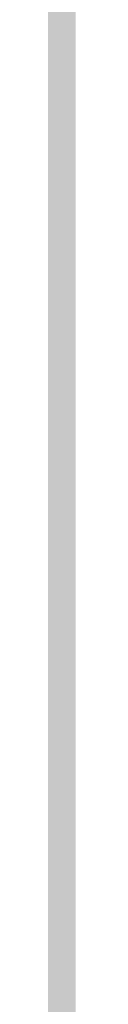
# Model space of a CAD drawing. Units: inches. Extents: x 2083 to 3317, y 1141 to 2115.
# Tile 208 of 256: x 3126.939 to 3126.956, y 1264.131 to 1265.165. Entities that reach past the tile are written whole.
import ezdxf

# ---------------------------------------------------------------- set-up
doc = ezdxf.new("R2010")
doc.units = ezdxf.units.IN
doc.layers.add('A-ANNO-DIMS', color=2, linetype='Continuous', lineweight=18)
doc.layers.add('A-WALL-PATT', color=251, linetype='Continuous', lineweight=13, true_color=0x636466)
doc.styles.get("Standard").update_dxf_attribs({"font": 'arial.ttf'})
doc.dimstyles.new('ISO-25', dxfattribs={"dimtxt": 12, "dimasz": 12, "dimexe": 1.25, "dimexo": 0.625, "dimtad": 1, "dimlunit": 3, "dimtxsty": 'Standard', "dimcen": 2.5, "dimadec": 0, "dimazin": 0, "dimtfac": 1, "dimtmove": 0, "dimatfit": 3, "dimfxl": 1, "dimarcsym": 0})

# ---------------------------------------------------------------- blocks, each defined once
blk = doc.blocks.new('*D26')
at = {"layer": 'A-ANNO-DIMS', "color": 0, "lineweight": -2, "transparency": 16777216}
for p, q in [((3088.9858, 1274.9151), (3088.9858, 1270.952)), ((3111.24, 1274.9151), (3111.24, 1270.952)), ((3076.9858, 1272.202), (2840.2624, 1272.202)), ((3111.24, 1272.202), (3088.9858, 1272.202)), ((3123.24, 1272.202), (3135.24, 1272.202))]:
    blk.add_line(p, q, dxfattribs=at)
at = {"layer": 'A-ANNO-DIMS', "color": 0, "transparency": 16777216}
for points in [[(3076.9858, 1274.202), (3076.9858, 1270.202), (3088.9858, 1272.202)], [(3123.24, 1274.202), (3123.24, 1270.202), (3111.24, 1272.202)]]:
    blk.add_solid(points, dxfattribs=at)
at = {"layer": 'Defpoints', "color": 0, "transparency": 16777216}
for p in [(3088.9858, 1275.5401), (3111.24, 1275.5401), (3088.9858, 1272.202)]:
    blk.add_point(p, dxfattribs=at)
at = {"layer": 'A-ANNO-DIMS', "color": 0, "transparency": 16777216, "insert": (2952.6241, 1279.0316), "char_height": 12, "attachment_point": 5}
blk.add_mtext('NIGHTSTAND 1\'-10 1/2" TYP.', dxfattribs=at)
blk = doc.blocks.new('*D27')
at = {"layer": 'A-ANNO-DIMS', "color": 0, "lineweight": -2, "transparency": 16777216}
for p, q in [((3114.5782, 1309.7943), (3114.5782, 1321.7943)), ((3111.865, 1297.7943), (3115.8282, 1297.7943)), ((3114.5782, 1297.7943), (3114.5782, 1275.5401)), ((3111.865, 1275.5401), (3115.8282, 1275.5401)), ((3114.5782, 1263.5401), (3114.5782, 1140.9886))]:
    blk.add_line(p, q, dxfattribs=at)
at = {"layer": 'A-ANNO-DIMS', "color": 0, "transparency": 16777216}
for points in [[(3112.5782, 1309.7943), (3116.5782, 1309.7943), (3114.5782, 1297.7943)], [(3112.5782, 1263.5401), (3116.5782, 1263.5401), (3114.5782, 1275.5401)]]:
    blk.add_solid(points, dxfattribs=at)
at = {"layer": 'Defpoints', "color": 0, "transparency": 16777216}
for p in [(3111.24, 1297.7943), (3111.24, 1275.5401), (3114.5782, 1275.5401)]:
    blk.add_point(p, dxfattribs=at)
at = {"layer": 'A-ANNO-DIMS', "color": 0, "transparency": 16777216, "insert": (3107.7485, 1196.2643), "char_height": 12, "attachment_point": 5, "rotation": 90}
blk.add_mtext('1\'-10 1/2" TYP.', dxfattribs=at)

msp = doc.modelspace()

# ---------------------------------------------------------------- hatches: boundary and pattern name
at = {"layer": 'A-WALL-PATT'}
h = msp.add_hatch(color=256, dxfattribs=at)
h.dxf.hatch_style = 1
h.paths.add_polyline_path([(3126.9598, 2020.7614), (2748.9598, 2020.7614), (2604.9598, 2020.7614), (2226.9598, 2020.7614), (2226.9598, 1702.7614), (2466.9598, 1702.7614), (2466.9598, 1582.7614), (2418.9598, 1582.7614), (2418.9598, 1477.7614), (2226.9598, 1477.7614), (2226.9598, 1263.2614), (2544.9598, 1263.2614), (2544.9598, 1411.7614), (2604.9598, 1411.7614), (2685.9598, 1411.7614), (2685.9598, 1420.7614), (2604.9598, 1420.7614), (2604.9598, 1573.7614), (2604.9598, 1702.7614), (2604.9598, 2011.7614), (2748.9598, 2011.7614), (2748.9598, 1702.7614), (2862.9598, 1702.7614), (2862.9598, 1621.7614), (2871.9598, 1621.7614), (2871.9598, 1702.7614), (2883.9598, 1702.7614), (2883.9598, 1706.9395, -0.026459), (2883.9598, 1711.7614), (2757.9598, 1711.7614), (2757.9598, 1807.7614), (2787.9598, 1807.7614), (2787.9598, 1812.2614), (2757.9598, 1812.2614), (2757.9598, 2011.7614), (2877.9598, 2011.7614), (2877.9598, 1812.2614), (2847.9598, 1812.2614), (2847.9598, 1807.7614), (2889.8357, 1807.7614), (2889.8357, 1812.2614), (2882.4598, 1812.2614), (2882.4598, 2011.7614), (3117.9598, 2011.7614), (3117.9598, 1812.2614), (2937.8357, 1812.2614), (2937.8357, 1807.7614), (2995.7098, 1807.7614), (2995.7098, 1796.1177), (3000.2098, 1796.1177), (3000.2098, 1807.7614), (3117.9598, 1807.7614), (3117.9598, 1711.7614), (3000.2098, 1711.7614), (3000.2098, 1760.1177), (2998.5727, 1760.1177, -0.020711), (2995.7098, 1760.1177), (2995.7098, 1711.7614), (2931.9598, 1711.7614), (2931.9598, 1702.7614), (3126.9598, 1702.7614)])
h.paths.add_polyline_path([(2471.4598, 2011.7614), (2471.4598, 1810.0114), (2462.7169, 1810.0114), (2462.7169, 1805.5114), (2505.9598, 1805.5114), (2505.9598, 1810.0114), (2475.9598, 1810.0114), (2475.9598, 2011.7614), (2595.9598, 2011.7614), (2595.9598, 1810.0114), (2565.9598, 1810.0114), (2565.9598, 1805.5114), (2595.9598, 1805.5114), (2595.9598, 1711.7614), (2235.9598, 1711.7614), (2235.9598, 1805.5114), (2353.7098, 1805.5114), (2353.7098, 1796.0542), (2358.2098, 1796.0542), (2358.2098, 1805.5114), (2414.7169, 1805.5114), (2414.7169, 1810.0114), (2235.9598, 1810.0114), (2235.9598, 2011.7614)], flags=16)
h.paths.add_polyline_path([(2270.2047, 1994.61), (2270.2047, 1970.61), (2246.2047, 1970.61), (2246.2047, 1994.61)], flags=0)
edge = h.paths.add_edge_path(flags=0)
edge.add_ellipse((2332.0274, 1899.7982), major_axis=(-3.043, 3.043), ratio=0.168252, start_angle=-161.3322, end_angle=-156.3071, ccw=False)
edge.add_ellipse((2333.082, 1898.7435), major_axis=(-1.0546, 1.0546), ratio=0.453532, start_angle=-123.371, end_angle=-94.1591)
edge = h.paths.add_edge_path(flags=0)
edge.add_ellipse((2332.0274, 1968.8763), major_axis=(3.043, 3.043), ratio=0.168252, start_angle=18.6678, end_angle=23.6929)
edge.add_spline(control_points=[(2332.9256, 1970.6911), (2332.2268, 1970.3361), (2330.8937, 1969.6589), (2328.4131, 1970.9321), (2327.2039, 1967.7487), (2324.7096, 1969.9556), (2322.5328, 1967.0124), (2320.0128, 1971.2958), (2317.6803, 1968.1578), (2316.0405, 1967.102), (2315.4269, 1966.8096)], knot_values=[0, 0, 0, 0, 2.267059, 4.324559, 6.685584, 8.878641, 11.121502, 14.300359, 17.755284, 19.732645, 19.732645, 19.732645, 19.732645], degree=3, periodic=0)
edge.add_ellipse((2332.0274, 1968.8763), major_axis=(3.043, 3.043), ratio=0.168252, start_angle=18.6678, end_angle=23.6929, ccw=False)
edge.add_ellipse((2333.082, 1969.9309), major_axis=(1.0546, 1.0546), ratio=0.453532, start_angle=56.629, end_angle=85.8409, ccw=False)
edge = h.paths.add_edge_path(flags=0)
edge.add_spline(control_points=[(2296.4283, 1967.9879), (2293.6278, 1965.3363), (2287.7036, 1959.7271), (2299.7439, 1949.9957), (2294.5326, 1935.6685), (2290.5732, 1920.6035), (2293.3941, 1909.9737), (2296.1854, 1904.9665)], knot_values=[0.099185, 0.099185, 0.099185, 0.099185, 0.345301, 0.619822, 0.982653, 1.386093, 1.810555, 1.810555, 1.810555, 1.810555], degree=3, periodic=0)
edge.add_spline(control_points=[(2296.1854, 1904.9665), (2297.3836, 1902.6193), (2298.001, 1901.9493), (2298.553, 1901.4682)], knot_values=[0.006246, 0.006246, 0.006246, 0.006246, 0.055476, 0.055476, 0.055476, 0.055476], degree=3, periodic=0)
edge.add_spline(control_points=[(2298.553, 1901.4682), (2297.2586, 1900.9232), (2295.2253, 1900.2321), (2293.0602, 1900.6142), (2292.1014, 1900.7884), (2292.0896, 1900.7906)], knot_values=[0.312835, 0.312835, 0.312835, 0.312835, 0.40178, 0.474987, 0.475903, 0.475903, 0.475903, 0.475903], degree=3, periodic=0)
edge.add_arc((2292.7936, 1904.6641), 3.937, 215.4209, 259.6982, ccw=False)
edge.add_spline(control_points=[(2289.5853, 1902.3823), (2289.4767, 1902.5351), (2289.3685, 1902.688), (2289.2609, 1902.8412)], knot_values=[0.102872, 0.102872, 0.102872, 0.102872, 0.116896, 0.116896, 0.116896, 0.116896], degree=3, periodic=0)
edge.add_spline(control_points=[(2289.2609, 1902.8412), (2288.6866, 1902.5502), (2287.64, 1902.0199), (2285.8813, 1901.874), (2283.853, 1901.5044), (2281.72, 1899.7105), (2278.467, 1899.4929), (2276.1571, 1901.8832), (2272.259, 1899.8041), (2267.7776, 1901.8432), (2262.2439, 1900.184), (2257.4149, 1901.7821), (2254.3184, 1900.7261), (2253.1783, 1900.3373)], knot_values=[0, 0, 0, 0, 1.907977, 3.477176, 5.261074, 7.972851, 11.680248, 13.717921, 16.939592, 22.789562, 27.502503, 33.595215, 37.145618, 37.145618, 37.145618, 37.145618], degree=3, periodic=0)
edge.add_line((2253.1783, 1900.3373), (2250.2442, 1902.8412))
edge.add_line((2250.2442, 1902.8412), (2250.2442, 1965.8333))
edge.add_line((2250.2442, 1965.8333), (2253.1783, 1968.3371))
edge.add_spline(control_points=[(2253.1783, 1968.3371), (2254.3184, 1967.9483), (2257.4149, 1966.8924), (2262.2439, 1968.4904), (2267.7776, 1966.8313), (2271.5267, 1968.5372), (2273.8759, 1967.8283), (2274.2067, 1967.7276)], knot_values=[0, 0, 0, 0, 0.09018, 0.244935, 0.364644, 0.513233, 0.537855, 0.537855, 0.537855, 0.537855], degree=3, periodic=0)
edge.add_arc((2274.3529, 1963.7933), 3.937, 72.0511, 92.1279, ccw=False)
edge.add_arc((2281.2969, 1985.23), 18.5963, 252.05113, 288.56572)
edge.add_arc((2292.3167, 1956.0289), 12.6461, 71.02679, 113.77822, ccw=False)
edge = h.paths.add_edge_path(flags=0)
edge.add_spline(control_points=[(2274.8994, 1951.8562), (2275.0662, 1951.6166), (2275.2327, 1951.3766), (2275.398, 1951.1359)], knot_values=[1.409916, 1.409916, 1.409916, 1.409916, 1.43159, 1.43159, 1.43159, 1.43159], degree=3, periodic=0)
edge.add_spline(control_points=[(2275.398, 1951.1359), (2275.7921, 1950.5619), (2276.1792, 1949.9838), (2276.5455, 1949.3971)], knot_values=[1.358238, 1.358238, 1.358238, 1.358238, 1.409916, 1.409916, 1.409916, 1.409916], degree=3, periodic=0)
edge.add_line((2276.5455, 1949.3971), (2277.4373, 1947.8622))
edge.add_spline(control_points=[(2277.4373, 1947.8622), (2276.3038, 1945.6731), (2274.6397, 1942.4269), (2274.6316, 1938.0939), (2272.7991, 1930.8515), (2274.3564, 1943.897), (2275.9477, 1947.9234), (2276.5455, 1949.3971)], knot_values=[0.005632, 0.005632, 0.005632, 0.005632, 0.186014, 0.266002, 0.357087, 0.59639, 0.739732, 0.739732, 0.739732, 0.739732], degree=3, periodic=0)
edge.add_spline(control_points=[(2276.5455, 1949.3971), (2276.1792, 1949.9838), (2275.7921, 1950.5619), (2275.398, 1951.1359)], knot_values=[1.358238, 1.358238, 1.358238, 1.358238, 1.409916, 1.409916, 1.409916, 1.409916], degree=3, periodic=0)
edge.add_spline(control_points=[(2275.398, 1951.1359), (2274.9425, 1950.0805), (2274.2078, 1948.0253), (2273.9346, 1944.8515), (2272.4685, 1937.6275), (2273.4662, 1945.6965), (2274.7006, 1951.0595), (2274.8994, 1951.8562)], knot_values=[0.104364, 0.104364, 0.104364, 0.104364, 0.189636, 0.269624, 0.36071, 0.600013, 0.644622, 0.644622, 0.644622, 0.644622], degree=3, periodic=0)
h.paths.add_polyline_path([(2269.1675, 1963.1276, -0.357527), (2268.1706, 1960.9764, -0.092561), (2268.1706, 1939.4363, -0.357527), (2269.1675, 1937.2851, -0.357527), (2267.0163, 1938.282, -0.164785), (2254.6856, 1938.282, -0.357527), (2252.5344, 1937.2851, -0.357527), (2253.5313, 1939.4363, -0.092561), (2253.5313, 1960.9764, -0.357527), (2252.5344, 1963.1276, -0.357527), (2254.6856, 1962.1307, -0.164785), (2267.0163, 1962.1307, -0.357527)], flags=0)
h.paths.add_polyline_path([(2248.8741, 1967.8018), (2248.8741, 1957.0277), (2249.4578, 1957.0277), (2249.4578, 1911.6468), (2248.8741, 1911.6468), (2248.8741, 1900.8727), (2246.5119, 1900.8727, 0.197327), (2244.1497, 1902.4569), (2244.1497, 1966.2176, 0.197327), (2246.5119, 1967.8018)], flags=0)
h.paths.add_polyline_path([(2269.1675, 1931.3893, -0.357527), (2268.1706, 1929.2381, -0.092561), (2268.1706, 1907.6981, -0.357527), (2269.1675, 1905.5469, -0.357527), (2267.0163, 1906.5438, -0.164785), (2254.6856, 1906.5438, -0.357527), (2252.5344, 1905.5469, -0.357527), (2253.5313, 1907.6981, -0.092561), (2253.5313, 1929.2381, -0.357527), (2252.5344, 1931.3893, -0.357527), (2254.6856, 1930.3925, -0.164785), (2267.0163, 1930.3925, -0.357527)], flags=0)
edge = h.paths.add_edge_path(flags=0)
edge.add_spline(control_points=[(2276.1969, 1906.7237), (2276.1681, 1909.0289), (2276.114, 1913.3719), (2270.5984, 1924.925), (2273.9052, 1919.0128), (2275.9217, 1916.2621), (2275.4746, 1912.4021), (2277.2579, 1910.3806), (2276.696, 1908.225), (2276.6462, 1906.813), (2276.6178, 1906.0084)], knot_values=[0, 0, 0, 0, 8.61026, 16.221274, 18.843057, 23.804898, 27.440828, 29.356102, 31.203478, 33.650687, 33.650687, 33.650687, 33.650687], degree=3, periodic=0)
edge.add_spline(control_points=[(2276.6178, 1906.0084), (2276.6233, 1905.6241), (2276.4977, 1904.6287), (2275.4418, 1903.8547), (2274.9373, 1903.0804), (2274.8591, 1902.8412)], knot_values=[0.156488, 0.156488, 0.156488, 0.156488, 0.184398, 0.231376, 0.250598, 0.250598, 0.250598, 0.250598], degree=3, periodic=0)
edge.add_line((2274.8591, 1902.8412), (2276.506, 1902.8412))
edge.add_spline(control_points=[(2276.506, 1902.8412), (2276.7883, 1903.0849), (2277.6651, 1904.1252), (2278.2495, 1904.3407), (2277.6539, 1908.5274), (2278.1557, 1906.2278), (2278.1005, 1905.2859), (2278.8467, 1904.069), (2277.8568, 1903.4149), (2277.8742, 1902.991), (2277.9036, 1902.8412)], knot_values=[0.059574, 0.059574, 0.059574, 0.059574, 0.080753, 0.103741, 0.16972, 0.176036, 0.207137, 0.240474, 0.262341, 0.27366, 0.27366, 0.27366, 0.27366], degree=3, periodic=0)
edge.add_line((2277.9036, 1902.8412), (2280.0298, 1902.8412))
edge.add_spline(control_points=[(2280.0298, 1902.8412), (2279.8882, 1903.0884), (2279.4993, 1903.9816), (2280.1523, 1905.9393), (2278.1036, 1909.6578), (2279.7624, 1907.1853), (2280.3279, 1904.8749), (2280.4851, 1903.4896), (2281.4633, 1903.2494), (2281.7583, 1902.9365), (2281.834, 1902.8412)], knot_values=[0.013856, 0.013856, 0.013856, 0.013856, 0.034874, 0.088867, 0.107879, 0.126738, 0.158714, 0.193757, 0.217487, 0.226722, 0.226722, 0.226722, 0.226722], degree=3, periodic=0)
edge.add_spline(control_points=[(2281.834, 1902.8412), (2281.7875, 1902.8267), (2281.647, 1902.783), (2281.3955, 1902.8595), (2281.0881, 1902.9852), (2280.7207, 1903.0609), (2280.3335, 1903.0257), (2280.1248, 1902.8989), (2280.0298, 1902.8412)], knot_values=[0, 0, 0, 0, 0.14413, 0.435517, 0.749276, 1.153046, 1.548371, 1.878348, 1.878348, 1.878348, 1.878348], degree=3, periodic=0)
edge.add_line((2280.0298, 1902.8412), (2277.9036, 1902.8412))
edge.add_spline(control_points=[(2277.9036, 1902.8412), (2277.8929, 1902.7959), (2277.8654, 1902.6796), (2277.6075, 1902.6875), (2277.2741, 1902.8007), (2276.8379, 1902.6198), (2276.5838, 1902.7893), (2276.506, 1902.8412)], knot_values=[0, 0, 0, 0, 0.127189, 0.326199, 0.628009, 1.24357, 1.515331, 1.515331, 1.515331, 1.515331], degree=3, periodic=0)
edge.add_line((2276.506, 1902.8412), (2274.8591, 1902.8412))
edge.add_spline(control_points=[(2274.8591, 1902.8412), (2274.8144, 1902.8986), (2274.7251, 1903.0134), (2274.4935, 1903.119), (2274.2443, 1902.9605), (2273.9371, 1903.1849), (2273.614, 1902.9831), (2273.4083, 1902.883), (2273.3223, 1902.8412)], knot_values=[0, 0, 0, 0, 0.21843, 0.436957, 0.687977, 0.990379, 1.398396, 1.69185, 1.69185, 1.69185, 1.69185], degree=3, periodic=0)
edge.add_spline(control_points=[(2273.3223, 1902.8412), (2273.6167, 1903.4457), (2274.274, 1904.5383), (2276.0272, 1904.5737), (2276.207, 1906.5836), (2276.1969, 1906.7237)], knot_values=[0.012227, 0.012227, 0.012227, 0.012227, 0.059472, 0.106218, 0.134458, 0.134458, 0.134458, 0.134458], degree=3, periodic=0)
h.paths.add_polyline_path([(2270.7761, 1897.7898), (2270.7761, 1873.7898), (2246.7761, 1873.7898), (2246.7761, 1897.7898)], flags=0)
h.paths.add_polyline_path([(2353.7098, 1760.0051), (2353.7098, 1760.0542), (2358.2098, 1760.0542, -0.033729)], flags=0)
h.paths.add_polyline_path([(2321.8191, 1737.5292), (2341.9953, 1737.5292, -0.414214), (2343.2033, 1736.3212), (2343.2033, 1721.0206, -0.414214), (2341.9953, 1719.8127), (2321.8191, 1719.8127, -0.414214), (2320.6112, 1721.0206), (2320.6112, 1736.3212, -0.414214)], flags=0)
h.paths.add_polyline_path([(2324.235, 1736.3212), (2339.5794, 1736.3212, -0.414214), (2341.9953, 1733.9053), (2341.9953, 1725.4497, -0.414214), (2339.5794, 1723.0338), (2333.6806, 1723.0338), (2333.8453, 1722.0455, -0.870646), (2335.4254, 1721.8259, -0.767327), (2333.9227, 1721.4232), (2331.291, 1721.4232, -0.767327), (2329.7883, 1721.8259, -0.870646), (2331.3684, 1722.0455), (2331.5331, 1723.0338), (2324.235, 1723.0338, -0.414214), (2321.8191, 1725.4497), (2321.8191, 1733.9053, -0.414214)], flags=0)
h.paths.add_polyline_path([(2570.4838, 1928.6154), (2589.6838, 1928.6154), (2590.1688, 1928.6154), (2590.1688, 1904.9934), (2570.4838, 1904.9934)], flags=0)
h.paths.add_polyline_path([(2574.4473, 1927.2638, -1), (2572.8288, 1927.2638, -1)], flags=0)
h.paths.add_polyline_path([(2573.0899, 1926.9409), (2573.925, 1927.776), (2574.1477, 1927.5533), (2573.3126, 1926.7182)], flags=0)
h.paths.add_polyline_path([(2578.7791, 1919.7296, -1), (2571.5917, 1919.7296, -1)], flags=0)
h.paths.add_polyline_path([(2578.3854, 1919.7296, -1), (2571.9854, 1919.7296, -1)], flags=0)
h.paths.add_polyline_path([(2331.5958, 1729.4762, -1), (2333.618, 1729.4762, -1)], flags=0)
h.paths.add_polyline_path([(2578.0342, 1927.2638, -1), (2576.4157, 1927.2638, -1)], flags=0)
h.paths.add_polyline_path([(2576.6889, 1927.5311), (2576.9116, 1927.7538), (2577.7467, 1926.9186), (2577.524, 1926.6959)], flags=0)
h.paths.add_polyline_path([(2578.1391, 1909.8595, -1), (2572.2317, 1909.8595, -1)], flags=0)
h.paths.add_polyline_path([(2577.7454, 1909.8595, -1), (2572.6254, 1909.8595, -1)], flags=0)
h.paths.add_polyline_path([(2583.7977, 1927.2638, -1), (2582.1792, 1927.2638, -1)], flags=0)
h.paths.add_polyline_path([(2582.7186, 1927.7538), (2583.5538, 1926.9186), (2583.3311, 1926.6959), (2582.4959, 1927.5311)], flags=0)
h.paths.add_polyline_path([(2582.4959, 1927.5311), (2582.7186, 1927.7538), (2583.5538, 1926.9186), (2583.3311, 1926.6959)], flags=0)
h.paths.add_polyline_path([(2587.7391, 1920.5296, -1), (2581.8317, 1920.5296, -1)], flags=0)
h.paths.add_polyline_path([(2587.3454, 1920.5296, -1), (2582.2254, 1920.5296, -1)], flags=0)
h.paths.add_polyline_path([(2587.3846, 1927.2638, -1), (2585.7661, 1927.2638, -1)], flags=0)
h.paths.add_polyline_path([(2586.082, 1926.9802), (2586.9172, 1927.8154), (2587.1399, 1927.5927), (2586.3047, 1926.7575)], flags=0)
h.paths.add_polyline_path([(2588.3791, 1910.6595, -1), (2581.1917, 1910.6595, -1)], flags=0)
h.paths.add_polyline_path([(2587.9854, 1910.6595, -1), (2581.5854, 1910.6595, -1)], flags=0)
h.paths.add_polyline_path([(2417.1677, 1729.4779), (2437.3439, 1729.4779, -0.414214), (2438.5519, 1728.2699), (2438.5519, 1712.9693, -0.414214), (2437.3439, 1711.7614), (2417.1677, 1711.7614, -0.414214), (2415.9598, 1712.9693), (2415.9598, 1728.2699, -0.414214)], flags=0)
h.paths.add_polyline_path([(2419.5836, 1728.2699), (2434.928, 1728.2699, -0.414214), (2437.3439, 1725.8541), (2437.3439, 1717.3984, -0.414214), (2434.928, 1714.9825), (2429.0292, 1714.9825), (2429.1939, 1713.9942, -0.870646), (2430.774, 1713.7746, -0.767327), (2429.2713, 1713.372), (2426.6396, 1713.372, -0.767327), (2425.1369, 1713.7746, -0.870646), (2426.717, 1713.9942), (2426.8817, 1714.9825), (2419.5836, 1714.9825, -0.414214), (2417.1677, 1717.3984), (2417.1677, 1725.8541, -0.414214)], flags=0)
h.paths.add_polyline_path([(2419.5836, 1728.2699), (2434.928, 1728.2699, -0.414214), (2437.3439, 1725.8541), (2437.3439, 1717.3984, -0.414214), (2434.928, 1714.9825), (2429.0292, 1714.9825), (2428.3581, 1719.009), (2427.5528, 1719.009), (2426.8817, 1714.9825), (2419.5836, 1714.9825, -0.414214), (2417.1677, 1717.3984), (2417.1677, 1725.8541, -0.414214)], flags=0)
h.paths.add_polyline_path([(2426.9444, 1721.4249, -1), (2428.9666, 1721.4249, -1)], flags=0)
h.paths.add_polyline_path([(2475.9598, 1702.7614), (2595.9598, 1702.7614), (2595.9598, 1582.7614), (2475.9598, 1582.7614)], flags=16)
h.paths.add_polyline_path([(2427.9598, 1573.7614), (2595.9598, 1573.7614), (2595.9598, 1468.7614), (2595.9598, 1420.7614), (2384.4598, 1420.7614), (2384.4598, 1468.7614), (2427.9598, 1468.7614)], flags=16)
h.paths.add_polyline_path([(2379.9598, 1468.7614), (2379.9598, 1420.7614), (2235.9598, 1420.7614), (2235.9598, 1468.7614)], flags=16)
h.paths.add_polyline_path([(2317.816, 1466.6958), (2337.9922, 1466.6958, -0.414214), (2339.2002, 1465.4878), (2339.2002, 1450.1872, -0.414214), (2337.9922, 1448.9792), (2317.816, 1448.9792, -0.414214), (2316.6081, 1450.1872), (2316.6081, 1465.4878, -0.414214)], flags=0)
h.paths.add_polyline_path([(2320.2319, 1465.4878), (2335.5763, 1465.4878, -0.414214), (2337.9922, 1463.0719), (2337.9922, 1454.6163, -0.414214), (2335.5763, 1452.2004), (2329.6775, 1452.2004), (2329.8422, 1451.212, -0.870646), (2331.4223, 1450.9925, -0.767327), (2329.9196, 1450.5898), (2327.2879, 1450.5898, -0.767327), (2325.7852, 1450.9925, -0.870646), (2327.3653, 1451.212), (2327.53, 1452.2004), (2320.2319, 1452.2004, -0.414214), (2317.816, 1454.6163), (2317.816, 1463.0719, -0.414214)], flags=0)
h.paths.add_polyline_path([(2320.2319, 1465.4878), (2335.5763, 1465.4878, -0.414214), (2337.9922, 1463.0719), (2337.9922, 1454.6163, -0.414214), (2335.5763, 1452.2004), (2329.6775, 1452.2004), (2329.0064, 1456.2269), (2328.2011, 1456.2269), (2327.53, 1452.2004), (2320.2319, 1452.2004, -0.414214), (2317.816, 1454.6163), (2317.816, 1463.0719, -0.414214)], flags=0)
h.paths.add_polyline_path([(2327.5926, 1458.6428, -1), (2329.6148, 1458.6428, -1)], flags=0)
h.paths.add_polyline_path([(2244.4117, 1433.3405), (2241.9209, 1433.3405, -0.414214), (2240.0179, 1435.2435), (2240.0179, 1440.9528, -0.414211), (2241.9209, 1442.8559), (2244.4117, 1442.8559, -1.976472)], flags=0)
h.paths.add_polyline_path([(2245.3569, 1434.3975, -0.414214), (2245.3569, 1441.7988, -2.144098)], flags=0)
h.paths.add_polyline_path([(2535.9598, 1416.2614), (2535.9598, 1272.2614), (2235.9598, 1272.2614), (2235.9598, 1416.2614)], flags=16)
h.paths.add_polyline_path([(2260.1196, 1384.2928), (2260.1196, 1362.0386), (2237.8654, 1362.0386), (2237.8654, 1384.2928)], flags=0)
edge = h.paths.add_edge_path(flags=0)
edge.add_line((2318.2518, 1362.0933), (2318.1458, 1362.001))
edge.add_ellipse((2317.4451, 1360.431), major_axis=(2.8216, 2.8216), ratio=0.168252, start_angle=18.6678, end_angle=20.9481, ccw=False)
edge.add_ellipse((2318.423, 1361.409), major_axis=(0.9779, 0.9779), ratio=0.453532, start_angle=56.629, end_angle=70.2262, ccw=False)
edge = h.paths.add_edge_path(flags=0)
edge.add_line((2319.1074, 1295.5711), (2319.015, 1295.6771))
edge.add_ellipse((2317.4451, 1296.3778), major_axis=(-2.8216, 2.8216), ratio=0.168252, start_angle=-161.3322, end_angle=-159.0519, ccw=False)
edge.add_ellipse((2318.423, 1295.3999), major_axis=(-0.9779, 0.9779), ratio=0.453532, start_angle=-123.371, end_angle=-109.7738)
edge = h.paths.add_edge_path(flags=0)
edge.add_spline(control_points=[(2284.2103, 1301.1702), (2284.5807, 1300.4447), (2284.8912, 1299.892), (2285.1596, 1299.461)], knot_values=[0.039066, 0.039066, 0.039066, 0.039066, 0.055476, 0.055476, 0.055476, 0.055476], degree=3, periodic=0)
edge.add_line((2285.1596, 1299.461), (2284.2103, 1301.1702))
edge = h.paths.add_edge_path(flags=0)
edge.add_line((2280.4125, 1297.298), (2283.37, 1297.0361))
edge.add_line((2283.37, 1297.0361), (2286.4057, 1297.9263))
edge.add_spline(control_points=[(2286.4057, 1297.9263), (2285.3055, 1297.4631), (2284.3448, 1297.1292), (2283.37, 1297.0361)], knot_values=[0.394369, 0.394369, 0.394369, 0.394369, 0.475903, 0.475903, 0.475903, 0.475903], degree=3, periodic=0)
edge.add_spline(control_points=[(2283.37, 1297.0361), (2283.2814, 1297.0277), (2282.3163, 1296.9573), (2281.3125, 1297.1345), (2280.4234, 1297.296), (2280.4125, 1297.298)], knot_values=[0.312835, 0.312835, 0.312835, 0.312835, 0.320246, 0.393453, 0.394369, 0.394369, 0.394369, 0.394369], degree=3, periodic=0)
edge = h.paths.add_edge_path(flags=0)
edge.add_line((2284.4356, 1359.6073), (2280.4463, 1355.328))
edge.add_line((2280.4463, 1355.328), (2279.58, 1351.0178))
edge.add_line((2279.58, 1351.0178), (2282.413, 1346.5804))
edge.add_spline(control_points=[(2282.413, 1346.5804), (2283.1533, 1345.5892), (2284.2529, 1344.0289), (2284.801, 1342.3872), (2284.9352, 1341.8055)], knot_values=[1.240098, 1.240098, 1.240098, 1.240098, 1.332892, 1.382712, 1.382712, 1.382712, 1.382712], degree=3, periodic=0)
edge.add_spline(control_points=[(2284.9352, 1341.8055), (2285.3191, 1340.1406), (2285.233, 1338.4092), (2284.9099, 1336.6541)], knot_values=[1.097484, 1.097484, 1.097484, 1.097484, 1.240098, 1.240098, 1.240098, 1.240098], degree=3, periodic=0)
edge.add_spline(control_points=[(2284.9099, 1336.6541), (2284.5868, 1334.899), (2284.0267, 1333.1203), (2283.4626, 1331.3606)], knot_values=[0.95487, 0.95487, 0.95487, 0.95487, 1.097484, 1.097484, 1.097484, 1.097484], degree=3, periodic=0)
edge.add_line((2283.4626, 1331.3606), (2281.8904, 1326.1534))
edge.add_line((2281.8904, 1326.1534), (2280.7563, 1321.0561))
edge.add_line((2280.7563, 1321.0561), (2280.2992, 1316.002))
edge.add_line((2280.2992, 1316.002), (2280.7159, 1310.9501))
edge.add_line((2280.7159, 1310.9501), (2282.0281, 1305.9721))
edge.add_line((2282.0281, 1305.9721), (2284.2103, 1301.1702))
edge.add_spline(control_points=[(2284.2103, 1301.1702), (2283.3407, 1302.7302), (2282.6119, 1304.3365), (2282.0281, 1305.9721)], knot_values=[0.099185, 0.099185, 0.099185, 0.099185, 0.241799, 0.241799, 0.241799, 0.241799], degree=3, periodic=0)
edge.add_spline(control_points=[(2282.0281, 1305.9721), (2281.4443, 1307.6078), (2281.0055, 1309.2728), (2280.7159, 1310.9501)], knot_values=[0.241799, 0.241799, 0.241799, 0.241799, 0.384413, 0.384413, 0.384413, 0.384413], degree=3, periodic=0)
edge.add_spline(control_points=[(2280.7159, 1310.9501), (2280.4332, 1312.5876), (2280.2894, 1314.277), (2280.2989, 1315.962), (2280.2992, 1316.002)], knot_values=[0.384413, 0.384413, 0.384413, 0.384413, 0.523647, 0.527028, 0.527028, 0.527028, 0.527028], degree=3, periodic=0)
edge.add_spline(control_points=[(2280.2992, 1316.002), (2280.3123, 1317.687), (2280.4779, 1319.3679), (2280.7563, 1321.0561)], knot_values=[0.527028, 0.527028, 0.527028, 0.527028, 0.669642, 0.669642, 0.669642, 0.669642], degree=3, periodic=0)
edge.add_spline(control_points=[(2280.7563, 1321.0561), (2281.0346, 1322.7443), (2281.4259, 1324.4396), (2281.8904, 1326.1534)], knot_values=[0.669642, 0.669642, 0.669642, 0.669642, 0.812256, 0.812256, 0.812256, 0.812256], degree=3, periodic=0)
edge.add_spline(control_points=[(2281.8904, 1326.1534), (2282.2644, 1327.5333), (2282.7879, 1329.2618), (2283.3528, 1331.0178), (2283.4626, 1331.3606)], knot_values=[0.812256, 0.812256, 0.812256, 0.812256, 0.927087, 0.95487, 0.95487, 0.95487, 0.95487], degree=3, periodic=0)
edge.add_line((2283.4626, 1331.3606), (2284.9099, 1336.6541))
edge.add_line((2284.9099, 1336.6541), (2284.9352, 1341.8055))
edge.add_line((2284.9352, 1341.8055), (2282.413, 1346.5804))
edge.add_spline(control_points=[(2282.413, 1346.5804), (2281.2751, 1348.1038), (2280.0784, 1349.5703), (2279.58, 1351.0178)], knot_values=[1.382712, 1.382712, 1.382712, 1.382712, 1.525326, 1.525326, 1.525326, 1.525326], degree=3, periodic=0)
edge.add_spline(control_points=[(2279.58, 1351.0178), (2279.4433, 1351.4147), (2279.1363, 1352.8569), (2279.7352, 1354.2904), (2280.4463, 1355.328)], knot_values=[1.525326, 1.525326, 1.525326, 1.525326, 1.564439, 1.667941, 1.667941, 1.667941, 1.667941], degree=3, periodic=0)
edge.add_spline(control_points=[(2280.4463, 1355.328), (2281.4261, 1356.7578), (2282.9308, 1358.1826), (2284.4356, 1359.6073)], knot_values=[1.667941, 1.667941, 1.667941, 1.667941, 1.810555, 1.810555, 1.810555, 1.810555], degree=3, periodic=0)
edge.add_arc((2280.6231, 1348.5182), 11.7262, 71.02679, 113.77822)
edge.add_arc((2270.4049, 1375.5952), 17.2436, 252.05113, 288.56572, ccw=False)
edge.add_arc((2263.966, 1355.7178), 3.6506, 72.0511, 92.1279)
edge.add_arc((2263.966, 1355.7178), 3.6506, 92.1279, 177.9851)
edge.add_spline(control_points=[(2260.3176, 1355.8462), (2260.2604, 1354.2207), (2260.5513, 1350.1865), (2262.9993, 1346.7663), (2264.4727, 1344.649)], knot_values=[1.43159, 1.43159, 1.43159, 1.43159, 1.564144, 1.770695, 1.770695, 1.770695, 1.770695], degree=3, periodic=0)
edge.add_line((2264.4727, 1344.649), (2264.9356, 1343.9825))
edge.add_spline(control_points=[(2263.801, 1340.2481), (2263.8432, 1340.5141), (2264.0672, 1341.7565), (2264.5127, 1343.0025), (2264.935, 1343.9811)], knot_values=[0.53657, 0.53657, 0.53657, 0.53657, 0.559349, 0.644622, 0.644622, 0.644622, 0.644622], degree=3, periodic=0)
edge.add_spline(control_points=[(2264.935, 1343.9811), (2265.1178, 1343.715), (2265.2989, 1343.4479), (2265.4768, 1343.1794)], knot_values=[1.384077, 1.384077, 1.384077, 1.384077, 1.409916, 1.409916, 1.409916, 1.409916], degree=3, periodic=0)
edge.add_spline(control_points=[(2265.4768, 1343.1794), (2265.6546, 1342.9108), (2265.8293, 1342.6408), (2265.9991, 1342.3688)], knot_values=[1.358238, 1.358238, 1.358238, 1.358238, 1.384077, 1.384077, 1.384077, 1.384077], degree=3, periodic=0)
edge.add_line((2265.9991, 1342.3688), (2266.826, 1340.9455))
edge.add_spline(control_points=[(2266.826, 1340.9455), (2268.8944, 1337.0897), (2271.3982, 1325.843), (2270.5162, 1310.5686), (2275.9194, 1301.8606), (2277.7895, 1299.1994)], knot_values=[0.116896, 0.116896, 0.116896, 0.116896, 0.472987, 1.050969, 1.313793, 1.313793, 1.313793, 1.313793], degree=3, periodic=0)
edge.add_spline(control_points=[(2277.7895, 1299.1994), (2277.8394, 1299.1285), (2277.8894, 1299.0575), (2277.9396, 1298.9866)], knot_values=[0.109884, 0.109884, 0.109884, 0.109884, 0.116896, 0.116896, 0.116896, 0.116896], degree=3, periodic=0)
edge.add_line((2277.9396, 1298.9866), (2277.7888, 1299.1991))
edge.add_spline(control_points=[(2277.7888, 1299.1991), (2277.2566, 1298.9294), (2276.2864, 1298.4379), (2275.0394, 1298.3344), (2274.3833, 1298.2389), (2274.2153, 1298.2093)], knot_values=[33.12187, 33.12187, 33.12187, 33.12187, 35.029056, 36.598255, 37.144827, 37.144827, 37.144827, 37.144827], degree=3, periodic=0)
edge.add_line((2274.2153, 1298.2093), (2273.0731, 1297.893))
edge.add_spline(control_points=[(2273.0731, 1297.893), (2272.3229, 1297.5798), (2271.0392, 1296.5105), (2269.2484, 1296.2261), (2268.4231, 1296.3747)], knot_values=[26.532584, 26.532584, 26.532584, 26.532584, 29.198919, 31.839101, 31.839101, 31.839101, 31.839101], degree=3, periodic=0)
edge.add_line((2268.4231, 1296.3747), (2263.8785, 1297.4575))
edge.add_spline(control_points=[(2263.8785, 1297.4575), (2263.5561, 1297.3594), (2261.8603, 1296.8387), (2260.2388, 1297.2824), (2258.9335, 1297.5165)], knot_values=[15.919551, 15.919551, 15.919551, 15.919551, 16.939592, 21.226067, 21.226067, 21.226067, 21.226067], degree=3, periodic=0)
edge.add_line((2258.9335, 1297.5165), (2254.0552, 1297.329))
edge.add_spline(control_points=[(2254.0552, 1297.329), (2253.7555, 1297.2958), (2252.1137, 1297.1652), (2250.4619, 1297.5442), (2249.1297, 1297.6679)], knot_values=[5.306517, 5.306517, 5.306517, 5.306517, 6.276435, 10.613034, 10.613034, 10.613034, 10.613034], degree=3, periodic=0)
edge.add_line((2249.1297, 1297.6679), (2244.3316, 1296.8778))
edge.add_line((2244.3316, 1296.8778), (2241.611, 1299.1994))
edge.add_line((2241.611, 1299.1994), (2241.611, 1357.6094))
edge.add_line((2241.611, 1357.6094), (2244.3316, 1359.9311))
edge.add_line((2244.3316, 1359.9311), (2252.7288, 1359.5427))
edge.add_spline(control_points=[(2252.7288, 1359.5427), (2252.8709, 1359.5464), (2253.3057, 1359.5482), (2253.7398, 1359.5143), (2254.0317, 1359.4824)], knot_values=[0.233291, 0.233291, 0.233291, 0.233291, 0.244935, 0.268927, 0.268927, 0.268927, 0.268927], degree=3, periodic=0)
edge.add_line((2254.0317, 1359.4824), (2259.5872, 1359.4164))
edge.add_spline(control_points=[(2259.5872, 1359.4164), (2260.6771, 1359.6285), (2262.0732, 1359.897), (2263.5237, 1359.4593), (2263.8304, 1359.366)], knot_values=[0.422516, 0.422516, 0.422516, 0.422516, 0.513233, 0.537855, 0.537855, 0.537855, 0.537855], degree=3, periodic=0)
edge.add_arc((2263.966, 1355.7178), 3.6506, 72.0511, 92.1279, ccw=False)
edge.add_arc((2270.4049, 1375.5952), 17.2436, 252.05113, 288.56572)
edge.add_arc((2280.6231, 1348.5182), 11.7262, 71.02679, 113.77822, ccw=False)
h.paths.add_polyline_path([(2240.3405, 1359.4347), (2240.3405, 1349.4444), (2240.8818, 1349.4444), (2240.8818, 1307.3645), (2240.3405, 1307.3645), (2240.3405, 1297.3741), (2238.1502, 1297.3741, 0.197327), (2235.9598, 1298.8431), (2235.9598, 1357.9657, 0.197327), (2238.1502, 1359.4347)], flags=0)
h.paths.add_polyline_path([(2259.1578, 1355.1005, -0.357527), (2258.2334, 1353.1058, -0.092561), (2258.2334, 1333.1326, -0.357527), (2259.1578, 1331.1379, -0.357527), (2257.1631, 1332.0622, -0.164785), (2245.7293, 1332.0622, -0.357527), (2243.7346, 1331.1379, -0.357527), (2244.6589, 1333.1326, -0.092561), (2244.6589, 1353.1058, -0.357527), (2243.7346, 1355.1005, -0.357527), (2245.7293, 1354.1761, -0.164785), (2257.1631, 1354.1761, -0.357527)], flags=0)
edge = h.paths.add_edge_path(flags=0)
edge.add_line((2265.9991, 1342.3688), (2266.826, 1340.9455))
edge.add_line((2266.826, 1340.9455), (2265.3076, 1337.8141))
edge.add_line((2265.3076, 1337.8141), (2264.3582, 1334.6529))
edge.add_line((2264.3582, 1334.6529), (2264.262, 1333.7997))
edge.add_spline(control_points=[(2264.262, 1333.7997), (2264.2084, 1333.1871), (2264.1621, 1332.3655), (2264.0071, 1331.4139), (2263.969, 1331.2018)], knot_values=[0.464444, 0.464444, 0.464444, 0.464444, 0.516691, 0.531608, 0.531608, 0.531608, 0.531608], degree=3, periodic=0)
edge.add_spline(control_points=[(2263.969, 1331.2018), (2263.7745, 1330.1189), (2263.4244, 1328.7908), (2263.2574, 1328.5307), (2263.234, 1328.5146)], knot_values=[0.372682, 0.372682, 0.372682, 0.372682, 0.44885, 0.464444, 0.464444, 0.464444, 0.464444], degree=3, periodic=0)
edge.add_spline(control_points=[(2263.234, 1328.5146), (2263.0964, 1328.4202), (2263.1312, 1329.3015), (2263.275, 1330.6157)], knot_values=[0.280919, 0.280919, 0.280919, 0.280919, 0.372682, 0.372682, 0.372682, 0.372682], degree=3, periodic=0)
edge.add_spline(control_points=[(2263.275, 1330.6157), (2263.4187, 1331.93), (2263.6715, 1333.6773), (2263.9699, 1335.315)], knot_values=[0.189157, 0.189157, 0.189157, 0.189157, 0.280919, 0.280919, 0.280919, 0.280919], degree=3, periodic=0)
edge.add_spline(control_points=[(2263.9699, 1335.315), (2264.1005, 1336.0322), (2264.4188, 1337.6219), (2264.7548, 1338.8644), (2264.9474, 1339.4911)], knot_values=[0.097394, 0.097394, 0.097394, 0.097394, 0.137578, 0.189157, 0.189157, 0.189157, 0.189157], degree=3, periodic=0)
edge.add_spline(control_points=[(2264.9474, 1339.4911), (2265.29, 1340.6061), (2265.6442, 1341.494), (2265.9991, 1342.3688)], knot_values=[0.005632, 0.005632, 0.005632, 0.005632, 0.097394, 0.097394, 0.097394, 0.097394], degree=3, periodic=0)
h.paths.add_polyline_path([(2259.1578, 1325.671, -0.357527), (2258.2334, 1323.6763, -0.092561), (2258.2334, 1303.7031, -0.357527), (2259.1578, 1301.7084, -0.357527), (2257.1631, 1302.6327, -0.164785), (2245.7293, 1302.6327, -0.357527), (2243.7346, 1301.7084, -0.357527), (2244.6589, 1303.7031, -0.092561), (2244.6589, 1323.6763, -0.357527), (2243.7346, 1325.671, -0.357527), (2245.7293, 1324.7466, -0.164785), (2257.1631, 1324.7466, -0.357527)], flags=0)
edge = h.paths.add_edge_path(flags=0)
edge.add_spline(control_points=[(2261.7089, 1317.3114), (2261.6795, 1317.4176), (2261.7619, 1317.3885), (2262.4907, 1316.0899), (2262.9622, 1315.3009)], knot_values=[14.955861, 14.955861, 14.955861, 14.955861, 16.221274, 18.694826, 18.694826, 18.694826, 18.694826], degree=3, periodic=0)
edge.add_spline(control_points=[(2262.9622, 1315.3009), (2262.9904, 1315.2536), (2263.7021, 1314.0674), (2264.349, 1313.1272), (2264.7301, 1312.1642)], knot_values=[18.694826, 18.694826, 18.694826, 18.694826, 18.843057, 22.433791, 22.433791, 22.433791, 22.433791], degree=3, periodic=0)
edge.add_spline(control_points=[(2264.7301, 1312.1642), (2264.8756, 1311.7964), (2265.1769, 1310.7698), (2265.1431, 1309.5593), (2265.2477, 1308.8242)], knot_values=[22.433791, 22.433791, 22.433791, 22.433791, 23.804898, 26.172756, 26.172756, 26.172756, 26.172756], degree=3, periodic=0)
edge.add_line((2265.2477, 1308.8242), (2265.8508, 1307.1719))
edge.add_spline(control_points=[(2265.8508, 1307.1719), (2266.065, 1306.8217), (2266.3844, 1306.3322), (2266.4244, 1305.7805), (2266.4204, 1305.6112)], knot_values=[28.062562, 28.062562, 28.062562, 28.062562, 29.356102, 29.911721, 29.911721, 29.911721, 29.911721], degree=3, periodic=0)
edge.add_spline(control_points=[(2266.4204, 1305.6112), (2266.4161, 1305.4326), (2266.394, 1305.25), (2266.3648, 1305.0659)], knot_values=[29.911721, 29.911721, 29.911721, 29.911721, 30.497837, 30.497837, 30.497837, 30.497837], degree=3, periodic=0)
edge.add_line((2266.3648, 1305.0659), (2266.0662, 1302.1363))
edge.add_spline(control_points=[(2266.0662, 1302.1363), (2266.0712, 1301.78), (2265.9981, 1301.2), (2265.6633, 1300.759), (2265.5089, 1300.5859)], knot_values=[0.156488, 0.156488, 0.156488, 0.156488, 0.184398, 0.203543, 0.203543, 0.203543, 0.203543], degree=3, periodic=0)
edge.add_line((2265.5089, 1300.5859), (2264.4353, 1299.1994))
edge.add_line((2264.4353, 1299.1994), (2265.9624, 1299.1994))
edge.add_line((2265.9624, 1299.1994), (2267.336, 1301.1753))
edge.add_line((2267.336, 1301.1753), (2267.3117, 1301.9862))
edge.add_spline(control_points=[(2267.3117, 1301.9862), (2267.2611, 1302.8624), (2267.1602, 1303.7371), (2267.2715, 1303.3259)], knot_values=[0.126229, 0.126229, 0.126229, 0.126229, 0.166617, 0.166617, 0.166617, 0.166617], degree=3, periodic=0)
edge.add_spline(control_points=[(2267.2715, 1303.3259), (2267.28, 1303.2943), (2267.3098, 1303.1754), (2267.3735, 1302.8836), (2267.4061, 1302.6828), (2267.4179, 1302.601)], knot_values=[0.166617, 0.166617, 0.166617, 0.166617, 0.16972, 0.176036, 0.180765, 0.180765, 0.180765, 0.180765], degree=3, periodic=0)
edge.add_spline(control_points=[(2267.7439, 1300.9875), (2267.6876, 1301.1509), (2267.4805, 1301.6567), (2267.4838, 1302.1448), (2267.4179, 1302.601)], knot_values=[0.180765, 0.180765, 0.180765, 0.180765, 0.193767, 0.220139, 0.220139, 0.220139, 0.220139], degree=3, periodic=0)
edge.add_line((2267.4179, 1302.601), (2267.7439, 1300.9875))
edge.add_spline(control_points=[(2267.7439, 1300.9875), (2267.832, 1300.7319), (2267.932, 1300.3099), (2267.5548, 1299.9745), (2267.4294, 1299.8292)], knot_values=[0.220139, 0.220139, 0.220139, 0.220139, 0.240474, 0.25489, 0.25489, 0.25489, 0.25489], degree=3, periodic=0)
edge.add_line((2267.4294, 1299.8292), (2267.2584, 1299.1994))
edge.add_line((2267.2584, 1299.1994), (2269.23, 1299.1994))
edge.add_spline(control_points=[(2269.23, 1299.1994), (2269.0987, 1299.4287), (2268.8428, 1300.0163), (2269.0116, 1300.9159), (2268.9468, 1301.6607)], knot_values=[0.013856, 0.013856, 0.013856, 0.013856, 0.034874, 0.067073, 0.067073, 0.067073, 0.067073], degree=3, periodic=0)
edge.add_line((2268.9468, 1301.6607), (2268.4316, 1303.6031))
edge.add_spline(control_points=[(2268.4316, 1303.6031), (2268.1756, 1304.1924), (2267.5962, 1305.2513), (2268.0407, 1304.6232), (2268.2514, 1304.2824)], knot_values=[0.090155, 0.090155, 0.090155, 0.090155, 0.107879, 0.120289, 0.120289, 0.120289, 0.120289], degree=3, periodic=0)
edge.add_spline(control_points=[(2268.2514, 1304.2824), (2268.3609, 1304.1053), (2269.0578, 1302.918), (2269.3827, 1301.5904), (2269.5214, 1300.7759), (2269.5752, 1300.5558)], knot_values=[0.120289, 0.120289, 0.120289, 0.120289, 0.126738, 0.158714, 0.173506, 0.173506, 0.173506, 0.173506], degree=3, periodic=0)
edge.add_line((2269.5752, 1300.5558), (2270.6858, 1299.4213))
edge.add_spline(control_points=[(2270.6858, 1299.4213), (2270.7672, 1299.3573), (2270.8379, 1299.2814), (2270.9029, 1299.1994)], knot_values=[0.21816, 0.21816, 0.21816, 0.21816, 0.226722, 0.226722, 0.226722, 0.226722], degree=3, periodic=0)
edge.add_line((2270.9372, 1299.1929), (2270.9029, 1299.1994))
edge.add_spline(control_points=[(2270.9029, 1299.1994), (2270.8598, 1299.186), (2270.7295, 1299.1455), (2270.4963, 1299.2164), (2270.2717, 1299.3083), (2270.121, 1299.348), (2270.0633, 1299.3596)], knot_values=[0.939174, 0.939174, 0.939174, 0.939174, 1.083304, 1.374691, 1.68845, 1.878348, 1.878348, 1.878348, 1.878348], degree=3, periodic=0)
edge.add_line((2270.0633, 1299.3596), (2269.23, 1299.1994))
edge.add_line((2269.23, 1299.1994), (2267.2584, 1299.1994))
edge.add_spline(control_points=[(2267.2584, 1299.1994), (2267.2484, 1299.1574), (2267.223, 1299.0497), (2266.9838, 1299.0569), (2266.8092, 1299.1162), (2266.6769, 1299.1091), (2266.6365, 1299.1048)], knot_values=[0.757665, 0.757665, 0.757665, 0.757665, 0.884854, 1.083864, 1.385675, 1.515331, 1.515331, 1.515331, 1.515331], degree=3, periodic=0)
edge.add_spline(control_points=[(2266.6365, 1299.1048), (2266.4852, 1299.0888), (2266.2358, 1299.0171), (2266.0346, 1299.1513), (2265.9624, 1299.1994)], knot_values=[0, 0, 0, 0, 0.485905, 0.757665, 0.757665, 0.757665, 0.757665], degree=3, periodic=0)
edge.add_line((2265.9624, 1299.1994), (2264.4353, 1299.1994))
edge.add_line((2264.4353, 1299.1994), (2263.8584, 1299.3671))
edge.add_spline(control_points=[(2263.8584, 1299.3671), (2263.8189, 1299.3709), (2263.7795, 1299.3857), (2263.7401, 1299.4015)], knot_values=[0.845925, 0.845925, 0.845925, 0.845925, 0.978627, 0.978627, 0.978627, 0.978627], degree=3, periodic=0)
edge.add_line((2263.7218, 1299.3964), (2263.0103, 1299.1994))
edge.add_spline(control_points=[(2263.0103, 1299.1994), (2263.2458, 1299.6829), (2263.506, 1300.1281), (2263.8735, 1300.408)], knot_values=[0.012227, 0.012227, 0.012227, 0.012227, 0.052971, 0.052971, 0.052971, 0.052971], degree=3, periodic=0)
edge.add_spline(control_points=[(2263.8735, 1300.408), (2263.9321, 1300.4527), (2264.0842, 1300.553), (2264.2552, 1300.6242), (2264.3597, 1300.6647)], knot_values=[0.052971, 0.052971, 0.052971, 0.052971, 0.059472, 0.069086, 0.069086, 0.069086, 0.069086], degree=3, periodic=0)
edge.add_line((2264.3597, 1300.6647), (2265.1419, 1301.0778))
edge.add_line((2265.1419, 1301.0778), (2265.6758, 1302.7996))
edge.add_line((2265.6758, 1302.7996), (2265.5407, 1305.7041))
edge.add_line((2265.5407, 1305.7041), (2264.8031, 1309.3277))
edge.add_line((2264.8031, 1309.3277), (2263.0405, 1314.0918))
edge.add_spline(control_points=[(2263.0405, 1314.0918), (2262.3836, 1315.6714), (2261.796, 1316.9977), (2261.7089, 1317.3114)], knot_values=[11.216896, 11.216896, 11.216896, 11.216896, 14.955861, 14.955861, 14.955861, 14.955861], degree=3, periodic=0)
h.paths.add_polyline_path([(2871.9598, 1416.2614), (2895.91, 1416.2614), (2895.91, 1420.7614), (2871.9598, 1420.7614), (2871.9598, 1501.7614), (2862.9598, 1501.7614), (2862.9598, 1420.7614), (2805.9598, 1420.7614), (2805.9598, 1411.7614), (2862.9598, 1411.7614), (2862.9598, 1263.2614), (3126.9598, 1263.2614), (3126.9598, 1411.7614), (3126.9598, 1486.7614), (2943.9598, 1486.7614), (2943.9598, 1477.7614), (2967.8603, 1477.7614), (2967.8603, 1420.7614), (2943.91, 1420.7614), (2943.91, 1416.2614), (3117.9598, 1416.2614), (3117.9598, 1420.7614), (2972.3603, 1420.7614), (2972.3603, 1477.7614), (3117.9598, 1477.7614), (3117.9598, 1420.7614), (3117.9598, 1272.2614), (2871.9598, 1272.2614)], flags=0)
h.paths.add_polyline_path([(2457.1256, 1485.9425), (2527.6027, 1485.9425), (2527.6027, 1537.6357), (2457.1256, 1537.6357)], flags=8)
h.paths.add_polyline_path([(2481.0051, 1609.9818), (2590.7658, 1609.9818), (2590.7658, 1682.0034), (2481.0051, 1682.0034)], flags=8)
h.paths.add_polyline_path([(2483.085, 1729.1268), (2553.562, 1729.1268), (2553.562, 1780.82), (2483.085, 1780.82)], flags=8)
h = msp.add_hatch(color=256, dxfattribs=at)
h.dxf.hatch_style = 1
h.paths.add_polyline_path([(3126.9598, 1486.7614), (2943.9598, 1486.7614), (2943.9598, 1477.7614), (2967.8603, 1477.7614), (2967.8603, 1420.7614), (2943.91, 1420.7614), (2943.91, 1416.2614), (3117.9598, 1416.2614), (3117.9598, 1420.7614), (2972.3603, 1420.7614), (2972.3603, 1477.7614), (3117.9598, 1477.7614), (3117.9598, 1420.7614), (3117.9598, 1272.2614), (2871.9598, 1272.2614), (2871.9598, 1416.2614), (2895.91, 1416.2614), (2895.91, 1420.7614), (2871.9598, 1420.7614), (2871.9598, 1501.7614), (2862.9598, 1501.7614), (2862.9598, 1420.7614), (2805.9598, 1420.7614), (2805.9598, 1411.7614), (2862.9598, 1411.7614), (2862.9598, 1263.2614), (3126.9598, 1263.2614), (3126.9598, 1411.7614)])

# ---------------------------------------------------------------- dimensions: what is measured, and where the dimension line sits
at = {"layer": 'A-ANNO-DIMS'}
for base, p1, p2, angle, text, picture, middle in [((3114.5782, 1275.5401), (3111.24, 1297.7943), (3111.24, 1275.5401), 270, '<> TYP.', '*D27', (3107.7485, 1196.2643)), ((3088.9858, 1272.202), (3111.24, 1275.5401), (3088.9858, 1275.5401), 180, 'NIGHTSTAND <> TYP.', '*D26', (2952.6241, 1279.0316))]:
    dim = msp.add_linear_dim(base=base, p1=p1, p2=p2, angle=angle, text=text, dimstyle='ISO-25', override={"dimdec": 1, "dimlfac": 1, "dimrnd": 0, "dimzin": 1, "dimdsep": 46, "dimlunit": 4, "dimfrac": 2}, dxfattribs=at)
    dim.commit()
    dim.dimension.update_dxf_attribs({"geometry": picture, "text_midpoint": middle})

doc.saveas('drawing.dxf')
